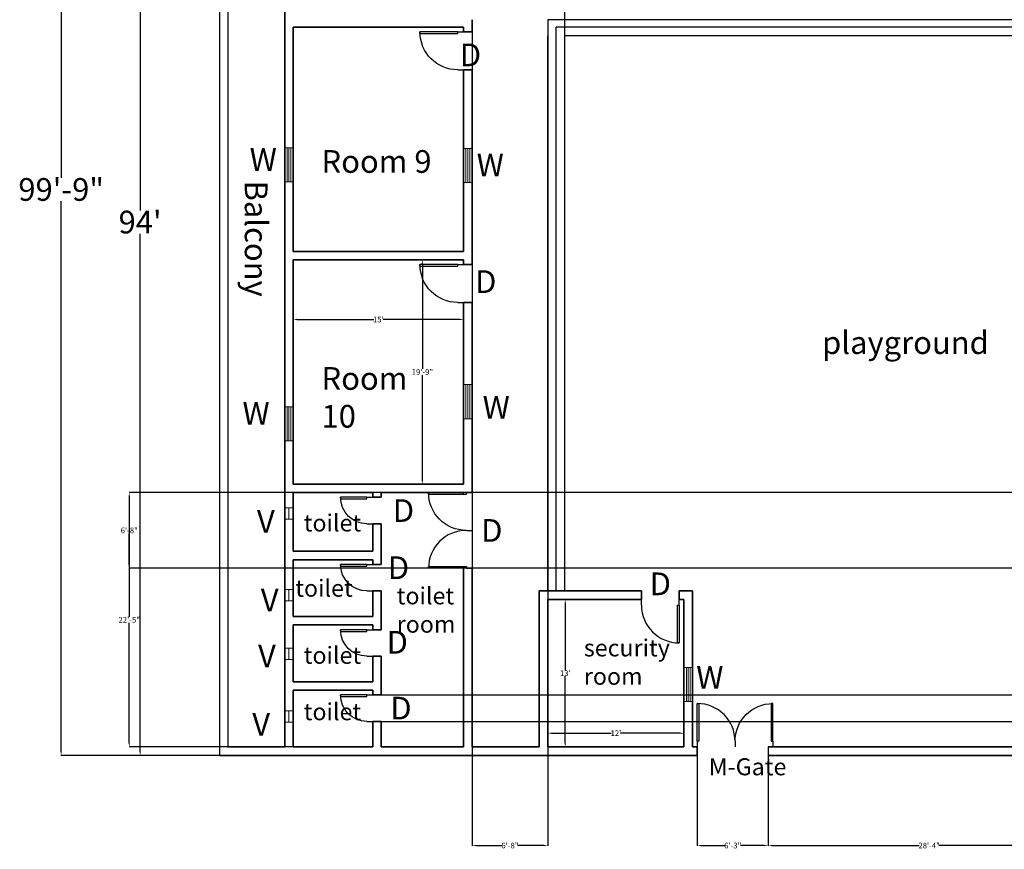
# Model space of a CAD drawing. Units: inches. Extents: x 6562 to 8578, y 2662 to 4218.
# Tile 1 of 3: x 6562 to 7603, y 2662 to 3539. Entities that reach past the tile are written whole.
import ezdxf

# ---------------------------------------------------------------- set-up
doc = ezdxf.new("R2010")
doc.units = ezdxf.units.IN
doc.header["$MEASUREMENT"] = 0
for name, color, linetype, lineweight in [('A-ANNO-DIMS', 2, 'Continuous', 18), ('A-ANNO-TEXT', 7, 'Continuous', 18), ('A-AREA-IDEN', 7, 'Continuous', 25), ('A-DOOR', 3, 'Continuous', 25), ('A-FLOR-EDGE', 8, 'Continuous', 25), ('A-GLAZ', 4, 'Continuous', 18), ('A-GLAZ-VENT', 4, 'Continuous', 18), ('A-WALL', 7, 'Continuous', 35)]:
    doc.layers.add(name, color=color, linetype=linetype, lineweight=lineweight)
doc.styles.get("Standard").update_dxf_attribs({"font": 'arial.ttf'})
doc.dimstyles.get("Standard").update_dxf_attribs({"dimtxt": 6, "dimasz": 4, "dimexe": 0.18, "dimexo": 0.0625, "dimgap": 0.09, "dimtad": 0, "dimtih": 1, "dimtoh": 1, "dimdec": 0, "dimzin": 0, "dimdsep": 46, "dimlunit": 3, "dimtxsty": 'Standard', "dimcen": 0.09, "dimadec": 0, "dimazin": 0, "dimtfac": 1, "dimtdec": 0, "dimtofl": 0, "dimtmove": 0, "dimatfit": 3, "dimfxl": 1, "dimtolj": 1, "dimtzin": 0, "dimarcsym": 0})

# ---------------------------------------------------------------- blocks, each defined once
blk = doc.blocks.new('*U3')
for p, q in [((-40, 0), (-40, 6)), ((0, 0), (0, 6))]:
    blk.add_line(p, q)
blk.add_lwpolyline([(0, 0), (0, -40), (-1.75, -40), (-1.75, 0)], close=True)
blk.add_arc((0, 0), 40, 180, 270)
blk = doc.blocks.new('*U2')
for p, q in [((0, 0), (0, -6)), ((40, 0), (40, -6))]:
    blk.add_line(p, q)
blk.add_lwpolyline([(0, 0), (0, 40), (1.75, 40), (1.75, 0)], close=True)
blk.add_arc((0, 0), 40, 0, 90)
blk = doc.blocks.new('*U6')
for p, q in [((0, 0), (0, -6)), ((28, 0), (28, -6))]:
    blk.add_line(p, q)
blk.add_lwpolyline([(0, 0), (0, 28), (1.75, 28), (1.75, 0)], close=True)
blk.add_arc((0, 0), 28, 0, 90)
blk = doc.blocks.new('*U7')
for p, q in [((0, 0), (0, -6)), ((40, 0), (40, -6))]:
    blk.add_line(p, q)
blk.add_lwpolyline([(0, 0), (0, 40), (1.75, 40), (1.75, 0)], close=True)
blk.add_arc((0, 0), 40, 0, 90)
blk = doc.blocks.new('*D13')
at = {"layer": 'A-ANNO-DIMS', "color": 0, "lineweight": -2, "transparency": 16777216}
for p, q in [((6773.1, 3958), (6605.8, 3958)), ((6606, 3954), (6606, 3371.8)), ((6606, 2765), (6606, 3347.2)), ((6773.1, 2761), (6605.8, 2761))]:
    blk.add_line(p, q, dxfattribs=at)
at = {"layer": 'A-ANNO-DIMS', "color": 0, "transparency": 16777216}
for points in [[(6605.3, 3954), (6606.6, 3954), (6606, 3958)], [(6605.3, 2765), (6606.6, 2765), (6606, 2761)]]:
    blk.add_solid(points, dxfattribs=at)
at = {"layer": 'Defpoints', "color": 0, "transparency": 16777216}
for p in [(6773.2, 3958), (6606, 2761), (6773.2, 2761)]:
    blk.add_point(p, dxfattribs=at)
at = {"layer": 'A-ANNO-DIMS', "color": 0, "transparency": 16777216, "insert": (6606, 3359.5), "char_height": 6, "attachment_point": 5}
blk.add_mtext('\\A1;{\\H4x;99\'-9"}', dxfattribs=at)
blk = doc.blocks.new('*D14')
at = {"layer": 'A-ANNO-DIMS', "color": 0, "lineweight": -2, "transparency": 16777216}
for p, q in [((6842.1, 3889), (6689.3, 3889)), ((6689.4, 3885), (6689.4, 3337.3)), ((6689.4, 2765), (6689.4, 3312.7)), ((6842.1, 2761), (6689.3, 2761))]:
    blk.add_line(p, q, dxfattribs=at)
at = {"layer": 'A-ANNO-DIMS', "color": 0, "transparency": 16777216}
for points in [[(6688.8, 3885), (6690.1, 3885), (6689.4, 3889)], [(6688.8, 2765), (6690.1, 2765), (6689.4, 2761)]]:
    blk.add_solid(points, dxfattribs=at)
at = {"layer": 'Defpoints', "color": 0, "transparency": 16777216}
for p in [(6842.2, 3889), (6689.4, 2761), (6842.2, 2761)]:
    blk.add_point(p, dxfattribs=at)
at = {"layer": 'A-ANNO-DIMS', "color": 0, "transparency": 16777216, "insert": (6689.4, 3325), "char_height": 6, "attachment_point": 5}
blk.add_mtext("\\A1;{\\H4x;94'}", dxfattribs=at)
blk = doc.blocks.new('*D15')
at = {"layer": 'A-ANNO-DIMS', "color": 0, "lineweight": -2, "transparency": 16777216}
for p, q in [((7120.2, 2926), (7138.8, 2926)), ((7138.7, 2922), (7138.7, 2851.2)), ((7138.7, 2774), (7138.7, 2844.8)), ((7120.2, 2770), (7138.8, 2770))]:
    blk.add_line(p, q, dxfattribs=at)
at = {"layer": 'A-ANNO-DIMS', "color": 0, "transparency": 16777216}
for points in [[(7138, 2922), (7139.3, 2922), (7138.7, 2926)], [(7138, 2774), (7139.3, 2774), (7138.7, 2770)]]:
    blk.add_solid(points, dxfattribs=at)
at = {"layer": 'Defpoints', "color": 0, "transparency": 16777216}
for p in [(7120.2, 2926), (7120.2, 2770), (7138.7, 2770)]:
    blk.add_point(p, dxfattribs=at)
at = {"layer": 'A-ANNO-DIMS', "color": 0, "transparency": 16777216, "insert": (7138.7, 2848), "char_height": 6, "attachment_point": 5}
blk.add_mtext("\\A1;13'", dxfattribs=at)
blk = doc.blocks.new('*D16')
at = {"layer": 'A-ANNO-DIMS', "color": 0, "lineweight": -2, "transparency": 16777216}
for p, q in [((7120.2, 2770.1), (7120.2, 2784.7)), ((7124.2, 2784.6), (7187.3, 2784.6)), ((7260.2, 2784.6), (7197.1, 2784.6)), ((7264.2, 2770.1), (7264.2, 2784.7))]:
    blk.add_line(p, q, dxfattribs=at)
at = {"layer": 'A-ANNO-DIMS', "color": 0, "transparency": 16777216}
for points in [[(7124.2, 2785.2), (7124.2, 2783.9), (7120.2, 2784.6)], [(7260.2, 2785.2), (7260.2, 2783.9), (7264.2, 2784.6)]]:
    blk.add_solid(points, dxfattribs=at)
at = {"layer": 'Defpoints', "color": 0, "transparency": 16777216}
for p in [(7264.2, 2784.6), (7120.2, 2770), (7264.2, 2770)]:
    blk.add_point(p, dxfattribs=at)
at = {"layer": 'A-ANNO-DIMS', "color": 0, "transparency": 16777216, "insert": (7192.2, 2784.6), "char_height": 6, "attachment_point": 5}
blk.add_mtext("\\A1;12'", dxfattribs=at)
blk = doc.blocks.new('*D19')
at = {"layer": 'A-ANNO-DIMS', "color": 0, "lineweight": -2, "transparency": 16777216}
for p, q in [((6941.2, 3285), (6987.9, 3285)), ((6987.7, 3281), (6987.7, 3169.7)), ((6987.7, 3052), (6987.7, 3163.3)), ((6941.2, 3048), (6987.9, 3048))]:
    blk.add_line(p, q, dxfattribs=at)
at = {"layer": 'A-ANNO-DIMS', "color": 0, "transparency": 16777216}
for points in [[(6987, 3281), (6988.3, 3281), (6987.7, 3285)], [(6987, 3052), (6988.3, 3052), (6987.7, 3048)]]:
    blk.add_solid(points, dxfattribs=at)
at = {"layer": 'Defpoints', "color": 0, "transparency": 16777216}
for p in [(6941.2, 3285), (6941.2, 3048), (6987.7, 3048)]:
    blk.add_point(p, dxfattribs=at)
at = {"layer": 'A-ANNO-DIMS', "color": 0, "transparency": 16777216, "insert": (6987.7, 3166.5), "char_height": 6, "attachment_point": 5}
blk.add_mtext('\\A1;19\'-9"', dxfattribs=at)
blk = doc.blocks.new('*D20')
at = {"layer": 'A-ANNO-DIMS', "color": 0, "lineweight": -2, "transparency": 16777216}
for p, q in [((6851.2, 3215.8), (6851.2, 3222.3)), ((6855.2, 3222.1), (6936.3, 3222.1)), ((7027.2, 3222.1), (6946.1, 3222.1)), ((7031.2, 3215.8), (7031.2, 3222.3))]:
    blk.add_line(p, q, dxfattribs=at)
at = {"layer": 'A-ANNO-DIMS', "color": 0, "transparency": 16777216}
for points in [[(6855.2, 3222.8), (6855.2, 3221.4), (6851.2, 3222.1)], [(7027.2, 3222.8), (7027.2, 3221.4), (7031.2, 3222.1)]]:
    blk.add_solid(points, dxfattribs=at)
at = {"layer": 'Defpoints', "color": 0, "transparency": 16777216}
for p in [(6851.2, 3215.8), (7031.2, 3222.1), (7031.2, 3215.8)]:
    blk.add_point(p, dxfattribs=at)
at = {"layer": 'A-ANNO-DIMS', "color": 0, "transparency": 16777216, "insert": (6941.2, 3222.1), "char_height": 6, "attachment_point": 5}
blk.add_mtext("\\A1;15'", dxfattribs=at)
blk = doc.blocks.new('VENT-12')
blk.add_line((4.5, 12), (4.5, 0))
blk.add_lwpolyline([(0, 12), (9, 12), (9, 0), (0, 0)], close=True)
blk = doc.blocks.new('WIN-36-OFFSET')
for p, q in [((2.5, 36), (2.5, 0)), ((4.5, 36), (4.5, 0)), ((6.5, 36), (6.5, 0))]:
    blk.add_line(p, q)
blk.add_lwpolyline([(0, 36), (9, 36), (9, 0), (0, 0)], close=True)
blk = doc.blocks.new('*D45')
at = {"layer": 'A-ANNO-DIMS', "color": 0, "lineweight": -2, "transparency": 16777216}
for p, q in [((7138.2, 2935.1), (7138.2, 4053.4)), ((7142.2, 4053.3), (7592.3, 4053.3)), ((8063.2, 4053.3), (7613, 4053.3)), ((8067.2, 3057.1), (8067.2, 4053.4))]:
    blk.add_line(p, q, dxfattribs=at)
at = {"layer": 'A-ANNO-DIMS', "color": 0, "transparency": 16777216}
for points in [[(7142.2, 4053.9), (7142.2, 4052.6), (7138.2, 4053.3)], [(8063.2, 4053.9), (8063.2, 4052.6), (8067.2, 4053.3)]]:
    blk.add_solid(points, dxfattribs=at)
at = {"layer": 'Defpoints', "color": 0, "transparency": 16777216}
for p in [(8067.2, 4053.3), (8067.2, 3057), (7138.2, 2935)]:
    blk.add_point(p, dxfattribs=at)
at = {"layer": 'A-ANNO-DIMS', "color": 0, "transparency": 16777216, "insert": (7602.7, 4053.3), "char_height": 6, "attachment_point": 5}
blk.add_mtext('\\A1;77\'-5"', dxfattribs=at)
blk = doc.blocks.new('*D47')
at = {"layer": 'A-ANNO-DIMS', "color": 0, "lineweight": -2, "transparency": 16777216}
for p, q in [((7040.2, 3538.9), (7040.2, 2665.6)), ((7120.2, 3538.9), (7120.2, 2665.6)), ((7044.2, 2665.8), (7072.1, 2665.8)), ((7116.2, 2665.8), (7088.3, 2665.8))]:
    blk.add_line(p, q, dxfattribs=at)
at = {"layer": 'A-ANNO-DIMS', "color": 0, "transparency": 16777216}
for points in [[(7044.2, 2666.4), (7044.2, 2665.1), (7040.2, 2665.8)], [(7116.2, 2666.4), (7116.2, 2665.1), (7120.2, 2665.8)]]:
    blk.add_solid(points, dxfattribs=at)
at = {"layer": 'Defpoints', "color": 0, "transparency": 16777216}
for p in [(7040.2, 3539), (7120.2, 3539), (7120.2, 2665.8)]:
    blk.add_point(p, dxfattribs=at)
at = {"layer": 'A-ANNO-DIMS', "color": 0, "transparency": 16777216, "insert": (7080.2, 2665.8), "char_height": 6, "attachment_point": 5}
blk.add_mtext('\\A1;6\'-8"', dxfattribs=at)
blk = doc.blocks.new('*D48')
at = {"layer": 'A-ANNO-DIMS', "color": 0, "lineweight": -2, "transparency": 16777216}
for p, q in [((7278.2, 2769.9), (7278.2, 2665.6)), ((7353.2, 2769.9), (7353.2, 2665.6)), ((7282.2, 2665.8), (7307.6, 2665.8)), ((7349.2, 2665.8), (7323.8, 2665.8))]:
    blk.add_line(p, q, dxfattribs=at)
at = {"layer": 'A-ANNO-DIMS', "color": 0, "transparency": 16777216}
for points in [[(7282.2, 2666.4), (7282.2, 2665.1), (7278.2, 2665.8)], [(7349.2, 2666.4), (7349.2, 2665.1), (7353.2, 2665.8)]]:
    blk.add_solid(points, dxfattribs=at)
at = {"layer": 'Defpoints', "color": 0, "transparency": 16777216}
for p in [(7278.2, 2770), (7353.2, 2770), (7353.2, 2665.8)]:
    blk.add_point(p, dxfattribs=at)
at = {"layer": 'A-ANNO-DIMS', "color": 0, "transparency": 16777216, "insert": (7315.7, 2665.8), "char_height": 6, "attachment_point": 5}
blk.add_mtext('\\A1;6\'-3"', dxfattribs=at)
blk = doc.blocks.new('*D49')
at = {"layer": 'A-ANNO-DIMS', "color": 0, "lineweight": -2, "transparency": 16777216}
for p, q in [((7353.2, 2769.9), (7353.2, 2665.6)), ((7693.2, 2769.9), (7693.2, 2665.6)), ((7357.2, 2665.8), (7512.7, 2665.8)), ((7689.2, 2665.8), (7533.6, 2665.8))]:
    blk.add_line(p, q, dxfattribs=at)
at = {"layer": 'A-ANNO-DIMS', "color": 0, "transparency": 16777216}
for points in [[(7357.2, 2666.4), (7357.2, 2665.1), (7353.2, 2665.8)], [(7689.2, 2666.4), (7689.2, 2665.1), (7693.2, 2665.8)]]:
    blk.add_solid(points, dxfattribs=at)
at = {"layer": 'Defpoints', "color": 0, "transparency": 16777216}
for p in [(7353.2, 2770), (7693.2, 2770), (7693.2, 2665.8)]:
    blk.add_point(p, dxfattribs=at)
at = {"layer": 'A-ANNO-DIMS', "color": 0, "transparency": 16777216, "insert": (7523.2, 2665.8), "char_height": 6, "attachment_point": 5}
blk.add_mtext('\\A1;28\'-4"', dxfattribs=at)
blk = doc.blocks.new('*D51')
at = {"layer": 'A-ANNO-DIMS', "color": 0, "lineweight": -2, "transparency": 16777216}
for p, q in [((6935.2, 2825), (8527.6, 2825)), ((8527.4, 2821), (8527.4, 2814.1)), ((8527.4, 2801), (8527.4, 2807.9)), ((6935.2, 2797), (8527.6, 2797))]:
    blk.add_line(p, q, dxfattribs=at)
at = {"layer": 'A-ANNO-DIMS', "color": 0, "transparency": 16777216}
for points in [[(8526.8, 2821), (8528.1, 2821), (8527.4, 2825)], [(8526.8, 2801), (8528.1, 2801), (8527.4, 2797)]]:
    blk.add_solid(points, dxfattribs=at)
at = {"layer": 'Defpoints', "color": 0, "transparency": 16777216}
for p in [(6935.2, 2825), (8527.4, 2825), (6935.2, 2797)]:
    blk.add_point(p, dxfattribs=at)
at = {"layer": 'A-ANNO-DIMS', "color": 0, "transparency": 16777216, "insert": (8527.4, 2811), "char_height": 6, "attachment_point": 5}
blk.add_mtext('\\A1;2\'-4"', dxfattribs=at)
blk = doc.blocks.new('*D57')
at = {"layer": 'A-ANNO-DIMS', "color": 0, "lineweight": -2, "transparency": 16777216}
for p, q in [((6851.1, 3039), (6677.7, 3039)), ((6677.9, 3035), (6677.9, 2907.7)), ((6677.9, 2774), (6677.9, 2901.3)), ((6851.1, 2770), (6677.7, 2770))]:
    blk.add_line(p, q, dxfattribs=at)
at = {"layer": 'A-ANNO-DIMS', "color": 0, "transparency": 16777216}
for points in [[(6677.3, 3035), (6678.6, 3035), (6677.9, 3039)], [(6677.3, 2774), (6678.6, 2774), (6677.9, 2770)]]:
    blk.add_solid(points, dxfattribs=at)
at = {"layer": 'Defpoints', "color": 0, "transparency": 16777216}
for p in [(6677.9, 3039), (6851.2, 3039), (6851.2, 2770)]:
    blk.add_point(p, dxfattribs=at)
at = {"layer": 'A-ANNO-DIMS', "color": 0, "transparency": 16777216, "insert": (6677.9, 2904.5), "char_height": 6, "attachment_point": 5}
blk.add_mtext('\\A1;22\'-5"', dxfattribs=at)
blk = doc.blocks.new('*D58')
at = {"layer": 'A-ANNO-DIMS', "color": 0, "lineweight": -2, "transparency": 16777216}
for p, q in [((7693.1, 3039), (6677.7, 3039)), ((6677.9, 3035), (6677.9, 3002.2)), ((6677.9, 2963), (6677.9, 2995.8)), ((7693.1, 2959), (6677.7, 2959))]:
    blk.add_line(p, q, dxfattribs=at)
at = {"layer": 'A-ANNO-DIMS', "color": 0, "transparency": 16777216}
for points in [[(6677.3, 3035), (6678.6, 3035), (6677.9, 3039)], [(6677.3, 2963), (6678.6, 2963), (6677.9, 2959)]]:
    blk.add_solid(points, dxfattribs=at)
at = {"layer": 'Defpoints', "color": 0, "transparency": 16777216}
for p in [(6677.9, 3039), (7693.2, 3039), (7693.2, 2959)]:
    blk.add_point(p, dxfattribs=at)
at = {"layer": 'A-ANNO-DIMS', "color": 0, "transparency": 16777216, "insert": (6677.9, 2999), "char_height": 6, "attachment_point": 5}
blk.add_mtext('\\A1;6\'-8"', dxfattribs=at)

msp = doc.modelspace()

# ---------------------------------------------------------------- linework, layer by layer
at = {"layer": 'A-DOOR'}
msp.add_line((7273.17, 2770), (7278.17, 2770), dxfattribs=at)
for points in [[(7273.17, 2761), (7278.17, 2761), (7278.17, 2770), (7273.17, 2770)], [(7358.17, 2770), (7353.17, 2770), (7353.17, 2761), (7358.17, 2761)]]:
    msp.add_lwpolyline(points, dxfattribs=at)
at = {"layer": 'A-FLOR-EDGE'}
for p, q in [((6773.18, 3958), (6773.18, 2761)), ((6782.18, 3949), (6782.18, 2770)), ((8085.18, 3539), (7120.18, 3539)), ((7120.18, 3539), (7120.18, 2770)), ((8076.18, 3531), (7129.17, 3531)), ((7129.17, 2935), (7129.17, 3531)), ((7120.17, 2935), (7120.17, 3522)), ((7120.18, 3522), (7120.17, 3522)), ((8067.18, 3522), (7138.17, 3522)), ((7138.17, 2935), (7138.17, 3522)), ((6782.18, 2770), (6842.18, 2770))]:
    msp.add_line(p, q, dxfattribs=at)
at = {"layer": 'A-GLAZ'}
for p, q in [((7264.17, 2854.23), (7264.17, 2818.23)), ((7273.17, 2854.23), (7264.17, 2854.23)), ((7266.67, 2854.23), (7266.67, 2818.23)), ((7268.67, 2854.23), (7268.67, 2818.23)), ((7270.67, 2854.23), (7270.67, 2818.23)), ((7273.17, 2818.23), (7273.17, 2854.23)), ((7264.17, 2818.23), (7273.17, 2818.23))]:
    msp.add_line(p, q, dxfattribs=at)
at = {"layer": 'A-WALL'}
for p, q in [((6842.18, 3889), (6842.18, 2770)), ((7040.18, 3539), (7040.18, 3526)), ((6851.18, 3531), (6851.18, 3294)), ((7031.18, 3531), (6851.18, 3531)), ((7031.18, 3531), (7031.18, 3526)), ((7040.18, 3531), (7040.18, 3531)), ((7031.18, 3526), (7040.18, 3526)), ((7031.18, 3486), (7031.18, 3486)), ((7031.18, 3486), (7040.18, 3486)), ((7031.18, 3486), (7031.18, 3294)), ((7040.18, 3486), (7040.18, 3280)), ((7031.18, 3294), (6851.18, 3294)), ((7031.18, 3285), (6851.18, 3285)), ((6851.18, 3285), (6851.18, 3048)), ((7031.18, 3285), (7031.18, 3280)), ((7031.18, 3280), (7040.18, 3280)), ((7031.18, 3240), (7040.18, 3240)), ((7031.18, 3240), (7031.18, 3048)), ((7040.18, 3240), (7040.18, 3039)), ((7031.18, 3048), (6851.18, 3048)), ((6851.18, 3039), (6851.18, 2977)), ((6935.18, 3039), (6851.18, 3039)), ((6935.18, 3039), (6935.18, 3034)), ((7031.18, 3039), (6944.18, 3039)), ((6944.18, 3039), (6944.18, 3034)), ((7031.18, 3039), (7031.18, 3037.25)), ((6935.18, 3034), (6935.18, 3034)), ((6935.18, 3034), (6944.18, 3034)), ((6935.18, 3006), (6944.18, 3006)), ((6935.18, 3006), (6935.18, 2977)), ((6944.18, 3006), (6944.18, 2977)), ((7031.18, 2999.12), (7031.18, 2998.89)), ((6851.18, 2977), (6935.18, 2977)), ((6944.18, 2977), (6944.18, 2963)), ((6851.18, 2968), (6935.18, 2968)), ((6851.18, 2968), (6851.18, 2908)), ((6935.18, 2968), (6935.18, 2963)), ((6935.18, 2963), (6944.18, 2963)), ((7031.18, 2959), (7031.18, 2770)), ((7040.18, 2959), (7040.18, 2770)), ((6935.18, 2935), (6935.18, 2935)), ((6935.18, 2935), (6944.18, 2935)), ((6935.18, 2935), (6935.18, 2908)), ((6944.18, 2935), (6944.18, 2894)), ((7219.17, 2935), (7111.17, 2935)), ((7111.17, 2935), (7111.17, 2770)), ((7219.17, 2926), (7219.17, 2935)), ((7259.17, 2926), (7259.17, 2935)), ((7273.17, 2935), (7259.17, 2935)), ((7273.17, 2770), (7273.17, 2935)), ((7120.17, 2770), (7120.17, 2926)), ((7219.17, 2926), (7120.17, 2926)), ((7120.17, 2926), (7120.17, 2770)), ((7264.17, 2926), (7259.17, 2926)), ((7264.17, 2770), (7264.17, 2926)), ((6851.18, 2908), (6935.18, 2908)), ((6851.18, 2899), (6935.18, 2899)), ((6851.18, 2899), (6851.18, 2839)), ((6935.18, 2899), (6935.18, 2894)), ((6935.18, 2894), (6944.18, 2894)), ((6935.18, 2866), (6944.18, 2866)), ((6935.18, 2866), (6935.18, 2839)), ((6944.18, 2825), (6944.18, 2866)), ((6851.18, 2839), (6935.18, 2839)), ((6851.18, 2830), (6935.18, 2830)), ((6851.18, 2830), (6851.18, 2770)), ((6935.18, 2830), (6935.18, 2825)), ((6935.18, 2825), (6944.18, 2825)), ((6935.18, 2797), (6944.18, 2797)), ((6935.18, 2797), (6935.18, 2770)), ((6944.18, 2797), (6944.18, 2770)), ((6851.18, 2770), (6935.18, 2770)), ((6944.18, 2770), (7031.18, 2770)), ((7040.18, 2770), (7111.17, 2770)), ((7120.17, 2770), (7264.17, 2770)), ((7353.17, 2770), (7693.18, 2770)), ((7581.18, 2770), (7428.18, 2770)), ((6773.18, 2761), (7278.17, 2761)), ((7278.17, 2761), (6773.18, 2761)), ((7595.18, 2761), (7353.17, 2761)), ((7353.17, 2761), (7595.18, 2761)), ((8432.18, 2761), (7595.18, 2761))]:
    msp.add_line(p, q, dxfattribs=at)

# ---------------------------------------------------------------- block references
at = {"layer": 'A-DOOR', "xscale": -1, "rotation": 90.00000000000384}
for name, p in [('*U7', (7025.18, 3526)), ('*U7', (7025.18, 3280)), ('*U2', (7034.18, 3039)), ('*U6', (6929.18, 3034)), ('*U6', (6929.18, 2963)), ('*U6', (6929.18, 2894)), ('*U6', (6929.18, 2825))]:
    msp.add_blockref(name, p, dxfattribs=at)
at = {"layer": 'A-DOOR', "rotation": 90.00000000000384}
msp.add_blockref('*U2', (7034.18, 2959), dxfattribs=at)
at = {"layer": 'A-DOOR'}
for name, p in [('*U3', (7259.17, 2920)), ('*U2', (7278.17, 2776))]:
    msp.add_blockref(name, p, dxfattribs=at)
at = {"layer": 'A-DOOR', "xscale": -1}
msp.add_blockref('*U2', (7358.17, 2776), dxfattribs=at)
at = {"layer": 'A-GLAZ'}
for p in [(6842.18, 3367.65), (7031.18, 3366.76), (7031.18, 3117.12), (6842.18, 3093.83)]:
    msp.add_blockref('WIN-36-OFFSET', p, dxfattribs=at)
at = {"layer": 'A-GLAZ-VENT'}
for p in [(6842.18, 3010.99), (6842.18, 3010.99), (6842.18, 2924.52), (6842.18, 2924.52), (6842.18, 2862.51), (6842.18, 2862.51), (6842.18, 2796.3), (6842.18, 2796.3)]:
    msp.add_blockref('VENT-12', p, dxfattribs=at)

# ---------------------------------------------------------------- texts
at = {"layer": 'A-ANNO-TEXT', "attachment_point": 1}
for s, width, insert, char_height in [('D', 32.1856, (7027.29, 3513.78), 24), ('W', 32.1856, (6805.16, 3403.16), 24), ('W', 32.1856, (7045.06, 3397.48), 24), ('D', 32.1856, (7043.43, 3274.04), 24), ('W', 32.1856, (6797.57, 3134.82), 24), ('W', 32.1856, (7051.36, 3141.19), 24), ('D', 32.1856, (6956.44, 3031.99), 24), ('V', 32.1856, (6812.88, 3020.46), 24), ('D', 32.1856, (7049.83, 3010.96), 24), ('D', 32.1856, (6951.18, 2971.55), 24), ('D', 32.1856, (7227.91, 2954.51), 24), ('V', 32.1856, (6816.94, 2937.39), 24), ('D', 32.1856, (6949.87, 2892.72), 24), ('V', 32.1856, (6814.01, 2878.34), 24), ('W', 32.1856, (7277.12, 2855.59), 24), ('D', 32.1856, (6953.81, 2823.09), 24), ('V', 32.1856, (6807.9, 2806.1), 24), ('M-Gate', 20.0644, (7290.33, 2758.1), 18)]:
    msp.add_mtext_dynamic_manual_height_columns(s, width=width, gutter_width=40, heights=[0], dxfattribs=dict(at, insert=insert, char_height=char_height))
at = {"layer": 'A-AREA-IDEN', "attachment_point": 1}
for s, width, gutter_width, insert, char_height in [('Room 9', 125.7129, 1, (6881.11, 3401.09), 24), ('playground', 33.181, 40, (7410.09, 3209.52), 24), ('Room 10', 125.7129, 1, (6881.11, 3171.68), 24), ('toilet', 20.0644, 40, (6862.3, 3015.93), 18), ('toilet', 20.0644, 40, (6853.33, 2946.93), 18), ('toilet room', 20.5479, 40, (6960.58, 2938.84), 18), ('security room', 20.0644, 40, (7158.37, 2883.78), 18), ('toilet', 20.0644, 40, (6862.3, 2875.98), 18), ('toilet', 20.0644, 40, (6862.3, 2816.3), 18)]:
    msp.add_mtext_dynamic_manual_height_columns(s, width=width, gutter_width=gutter_width, heights=[0], dxfattribs=dict(at, insert=insert, char_height=char_height))
at = {"layer": 'A-AREA-IDEN', "insert": (6824.06, 3368.94), "char_height": 24, "attachment_point": 1, "rotation": 270}
msp.add_mtext_dynamic_manual_height_columns('Balcony', width=33.181, gutter_width=40, heights=[0], dxfattribs=at)

# ---------------------------------------------------------------- dimensions: what is measured, and where the dimension line sits
at = {"layer": 'A-ANNO-DIMS'}
for base, p1, p2, override, picture, middle in [((8067.18, 4053.25), (7138.17, 2935), (8067.18, 3057), {"dimdec": 1, "dimlfac": 1, "dimrnd": 0, "dimzin": 1, "dimdsep": 46, "dimlunit": 4, "dimfrac": 2}, '*D45', (7602.68, 4053.25)), ((7120.18, 2665.75), (7040.18, 3539), (7120.18, 3539), {"dimdec": 1, "dimlfac": 1, "dimrnd": 0, "dimzin": 1, "dimdsep": 46, "dimlunit": 4, "dimfrac": 2}, '*D47', (7080.18, 2665.75)), ((7031.18, 3222.08), (6851.18, 3215.77), (7031.18, 3215.77), {"dimclrd": 0, "dimclre": 0, "dimclrt": 0}, '*D20', (6941.18, 3222.08)), ((7264.17, 2784.56), (7120.17, 2770), (7264.17, 2770), {"dimclrd": 0, "dimclre": 0, "dimclrt": 0}, '*D16', (7192.17, 2784.56)), ((7353.17, 2665.75), (7278.17, 2770), (7353.17, 2770), {"dimdec": 1, "dimlfac": 1, "dimrnd": 0, "dimzin": 1, "dimdsep": 46, "dimlunit": 4, "dimfrac": 2}, '*D48', (7315.67, 2665.75)), ((7693.18, 2665.75), (7353.17, 2770), (7693.18, 2770), {"dimdec": 1, "dimlfac": 1, "dimrnd": 0, "dimzin": 1, "dimdsep": 46, "dimlunit": 4, "dimfrac": 2}, '*D49', (7523.18, 2665.75))]:
    dim = msp.add_linear_dim(base=base, p1=p1, p2=p2, dimstyle='Standard', override=override, dxfattribs=at)
    dim.commit()
    dim.dimension.update_dxf_attribs({"geometry": picture, "text_midpoint": middle})
for base, p1, p2, picture, middle in [((6605.96, 2761), (6773.18, 3958), (6773.18, 2761), '*D13', (6605.96, 3359.5)), ((6689.45, 2761), (6842.18, 3889), (6842.18, 2761), '*D14', (6689.45, 3325))]:
    dim = msp.add_linear_dim(base=base, p1=p1, p2=p2, angle=90, text='{\\H4x;<>}', dimstyle='Standard', override={"dimclrd": 0, "dimclre": 0, "dimclrt": 0}, dxfattribs=at)
    dim.commit()
    dim.dimension.update_dxf_attribs({"geometry": picture, "text_midpoint": middle})
for base, p1, p2, override, picture, middle in [((6987.68, 3048), (6941.18, 3285), (6941.18, 3048), {"dimclrd": 0, "dimclre": 0, "dimclrt": 0}, '*D19', (6987.68, 3166.5)), ((6677.93, 3039), (6851.18, 2770), (6851.18, 3039), {"dimdec": 1, "dimlfac": 1, "dimrnd": 0, "dimzin": 1, "dimdsep": 46, "dimlunit": 4, "dimfrac": 2}, '*D57', (6677.93, 2904.5)), ((6677.93, 3039), (7693.18, 2959), (7693.18, 3039), {"dimdec": 1, "dimlfac": 1, "dimrnd": 0, "dimzin": 1, "dimdsep": 46, "dimlunit": 4, "dimfrac": 2}, '*D58', (6677.93, 2999)), ((7138.66, 2770), (7120.17, 2926), (7120.17, 2770), {"dimclrd": 0, "dimclre": 0, "dimclrt": 0}, '*D15', (7138.66, 2848)), ((8527.43, 2825), (6935.18, 2797), (6935.18, 2825), {"dimdec": 1, "dimlfac": 1, "dimrnd": 0, "dimzin": 1, "dimdsep": 46, "dimlunit": 4, "dimfrac": 2}, '*D51', (8527.43, 2811))]:
    dim = msp.add_linear_dim(base=base, p1=p1, p2=p2, angle=90, dimstyle='Standard', override=override, dxfattribs=at)
    dim.commit()
    dim.dimension.update_dxf_attribs({"geometry": picture, "text_midpoint": middle})

doc.saveas('drawing.dxf')
